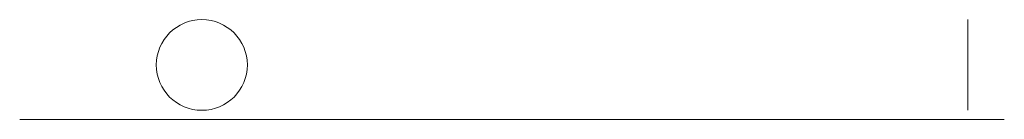
# Model space of a CAD drawing. Units: millimetres. Extents: x 908.9 to 963, y 235.1 to 240.6.
import ezdxf

# ---------------------------------------------------------------- set-up
doc = ezdxf.new("R2010")
doc.units = ezdxf.units.MM
doc.layers.add('M-CONS', color=8, linetype='Continuous', lineweight=18)

msp = doc.modelspace()

# ---------------------------------------------------------------- linework, layer by layer
at = {"layer": 'M-CONS', "extrusion": (0, -1, 0)}
for p, q in [((911.899, 235.09, -24.352), (911.899, 235.09, -2.141)), ((922.899, 235.09, -9.352), (914.899, 235.09, -9.352)), ((914.899, 235.09, -24.352), (914.899, 235.09, -9.352)), ((922.899, 235.09, -24.352), (922.899, 235.09, -9.352)), ((925.899, 235.09, -24.352), (925.899, 235.09, -2.141)), ((927.559, 235.09, 10), (952.959, 235.09, 10)), ((927.559, 235.09), (952.959, 235.09)), ((939.959, 235.09, 7), (952.959, 235.09, 7)), ((952.959, 235.09, 3), (939.959, 235.09, 3)), ((952.959, 235.09, 15), (952.959, 235.09, 10)), ((952.959, 235.09), (952.959, 235.09, -5)), ((952.959, 235.09, 15), (957.959, 235.09, 15)), ((952.959, 235.09, -5), (957.959, 235.09, -5)), ((957.959, 235.09, 15), (957.959, 235.09, 14)), ((957.959, 235.09, -4), (957.959, 235.09, -5)), ((959.959, 235.09, 12), (962.959, 235.09, 12)), ((962.959, 235.09, -2), (959.959, 235.09, -2)), ((962.959, 235.09, 9), (960.959, 235.09, 9)), ((960.959, 235.09, 9), (960.959, 235.09, 1)), ((960.959, 235.09, 1), (962.959, 235.09, 1)), ((960.959, 235.09, 1), (960.959, 235.09, 5)), ((962.959, 235.09, 12), (962.959, 235.09, 9)), ((962.959, 235.09, 1), (962.959, 235.09, -2))]:
    msp.add_line(p, q, dxfattribs=at)
at = {"layer": 'M-CONS', "extrusion": (0, 0, -1)}
msp.add_line((922.899, 235.09, -9.352), (918.899, 235.09, -9.352), dxfattribs=at)
at = {"layer": 'M-CONS', "extrusion": (0, -1, 0), "elevation": -235.09}
for points in [[(909.899, -29.352, -0.414214), (911.899, -31.352), (911.899, -34.352), (912.899, -34.352, 0.414214), (914.899, -32.352), (914.899, -29.352)], [(922.899, -29.352), (922.899, -32.352, 0.414214), (924.899, -34.352), (925.899, -34.352), (925.899, -31.352, -0.414214), (927.899, -29.352)]]:
    msp.add_lwpolyline(points, format="xyb", dxfattribs=at)
at = {"layer": 'M-CONS', "extrusion": (0, 0, -1)}
msp.add_circle((-918.899, 238.09, 9.352), 2.5, dxfattribs=at)
at = {"layer": 'M-CONS', "extrusion": (1, 0, 0)}
msp.add_circle((238.09, 5, 960.959), 2.5, dxfattribs=at)
at = {"layer": 'M-CONS', "extrusion": (0, -1, 0)}
msp.add_circle((918.899, 5, -235.09), 8, dxfattribs=at)
for centre, radius, start, end in [((918.899, 5, -235.09), 10, 30, 330), ((939.959, 5, -235.09), 2, 90, 270), ((952.959, 5, -235.09), 2, 270, 90), ((959.959, 14, -235.09), 2, 180, 270), ((959.959, -4, -235.09), 2, 90, 180)]:
    msp.add_arc(centre, radius, start, end, dxfattribs=at)

doc.saveas('drawing.dxf')
